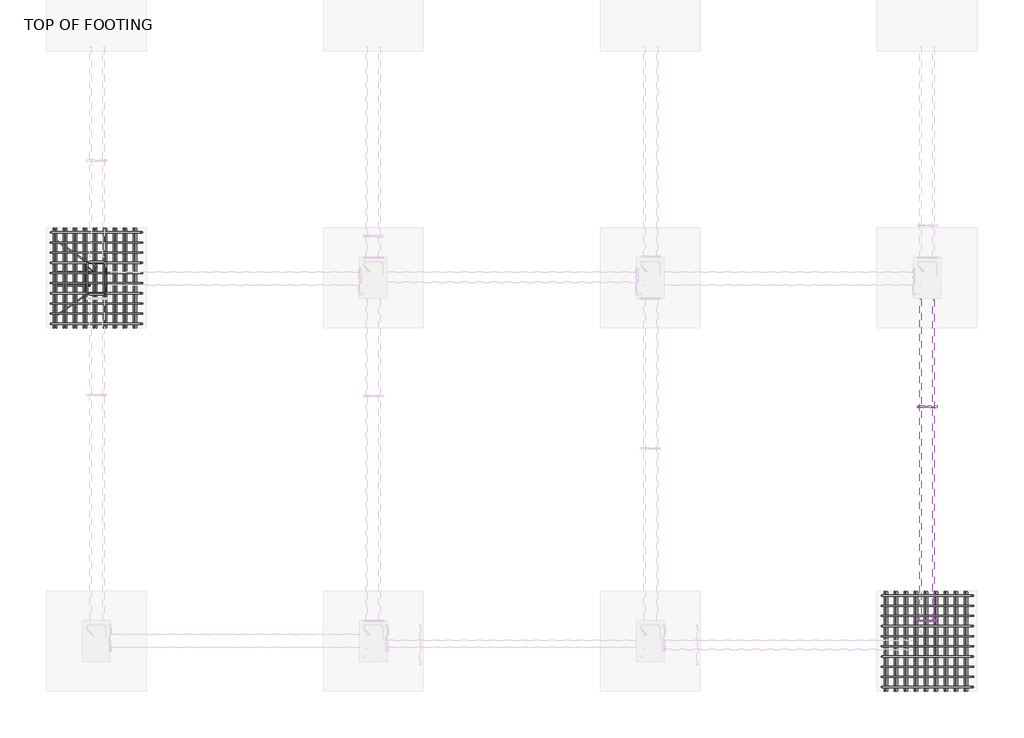
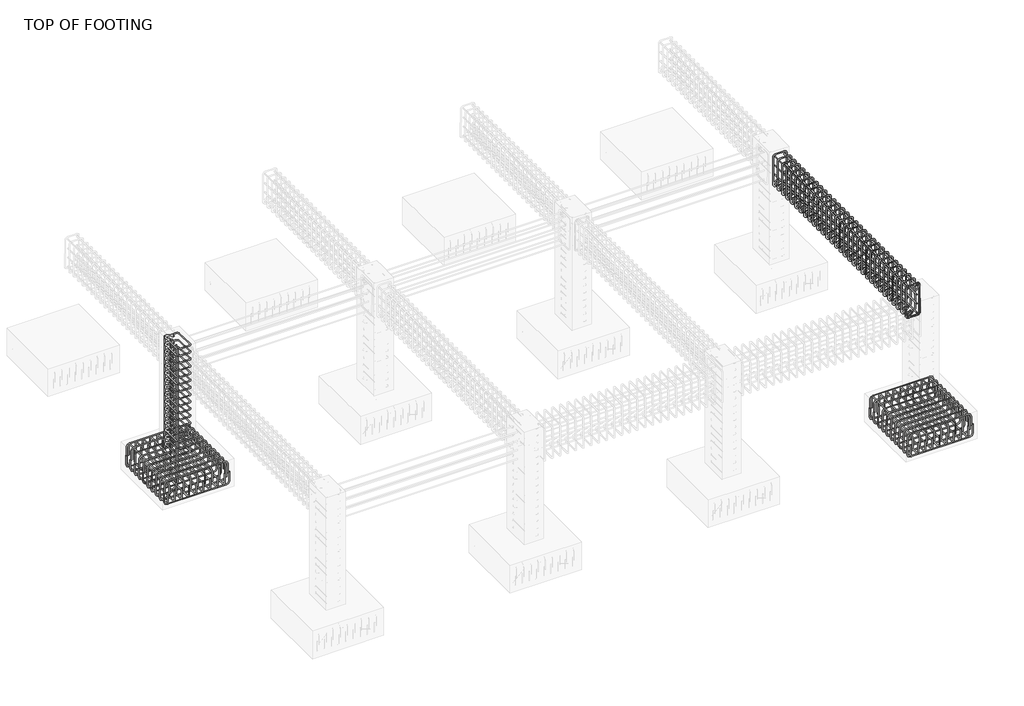
# One storey, part 5 of 18: 17 reinforcing bars.
"""IFC4 building model written with IfcOpenShell, lengths in millimetres."""

from ifc_helpers import new_model, si_unit, point, frame, origin, place, context, project, spatial, polyline, circle_curve, trimmed, segment, composite_curve, source, transform, mapped, element, save
from ifc_brep_helpers import swept_disk

model = new_model("IFC4")

# Units and contexts
model_context = context("Model", 3, world=origin())
ifc_project = project(units=[si_unit("LENGTHUNIT", "METRE", prefix="MILLI")], contexts=[model_context])

# Site, building, storey
site = spatial("IfcSite", under=ifc_project)
building = spatial("IfcBuilding", under=site)
storey = spatial("IfcBuildingStorey", under=building, Name="TOP OF FOOTING", Elevation=-1828.8)

# Reinforcing bars
placement = place(None, origin())
reinforcing_bar_shape = source(origin(), model_context, "Body", "SolidModel", [
    swept_disk(composite_curve([segment(polyline([(-11115.9859643, 9574.8477614, -40.0), (-11115.9859643, 9574.8477614, -2185.2530621)]), True, "CONTINUOUS"), segment(trimmed(circle_curve(frame((-11162.3359643, 9574.8477614, -2185.2530621), z_axis=(0.0, 1.0, 0.0), x_axis=(46.350000000000364, 0.0, 0.0)), 46.35), [point((-11115.9859643, 9574.8477614, -2185.2530621))], [point((-11162.3359643, 9574.8477614, -2231.6030621))], True, "CARTESIAN"), True, "CONTINUOUS"), segment(polyline([(-11162.3359643, 9574.8477614, -2231.6030621), (-11513.5126143, 9574.8477614, -2231.6030621)]), True, "CONTINUOUS")], self_intersect=False), 6.35),
])
element("IfcReinforcingBar", 1, at=placement, inside=storey, context=model_context, shape_type="MappedRepresentation", body=[
    mapped(reinforcing_bar_shape, transform((0.0, 0.0, 0.0), x_axis=(1.0, 0.0, 0.0), y_axis=(0.0, 1.0, 0.0), z_axis=(0.0, 0.0, 1.0))),
    mapped(reinforcing_bar_shape, transform((0.0, 148.3194112, 0.0), x_axis=(1.0, 0.0, 0.0), y_axis=(0.0, 1.0, 0.0), z_axis=(0.0, 0.0, 1.0))),
])
element("IfcReinforcingBar", 2, at=placement, inside=storey, context=model_context, shape_type="SolidModel", body=[
    swept_disk(composite_curve([segment(polyline([(-11140.9859643, 9830.3098681, -40.0), (-11140.9859643, 9830.3098681, -2185.2530621)]), True, "CONTINUOUS"), segment(trimmed(circle_curve(frame((-11178.9536616, 9856.895136, -2185.2530621), z_axis=(0.5735764363510552, 0.8191520442889855, 0.0), x_axis=(37.96769730000051, -26.585267899999963, 0.0)), 46.35), [point((-11140.9859643, 9830.3098681, -2185.2530621))], [point((-11178.9536616, 9856.895136, -2231.6030621))], True, "CARTESIAN"), True, "CONTINUOUS"), segment(polyline([(-11178.9536616, 9856.895136, -2231.6030621), (-11466.6207323, 10058.3217874, -2231.6030621)]), True, "CONTINUOUS")], self_intersect=False), 6.35),
])
reinforcing_bar_2_shape = source(origin(), model_context, "Body", "SolidModel", [
    swept_disk(composite_curve([segment(polyline([(-11036.6954038, 9770.3841028, -1782.45), (-11092.4389667, 9826.1276657, -1782.45)]), True, "CONTINUOUS"), segment(trimmed(circle_curve(frame((-11114.6067643, 9803.9598681, -1782.45), z_axis=(0.0, 0.0, 1.0), x_axis=(22.167797600000995, 22.167797599999176, 0.0)), 31.35), [point((-11092.4389667, 9826.1276657, -1782.45))], [point((-11145.9567643, 9803.9598681, -1782.45))], True, "CARTESIAN"), True, "CONTINUOUS"), segment(polyline([(-11145.9567643, 9803.9598681, -1782.45), (-11145.9567643, 9509.3598681, -1782.45)]), True, "CONTINUOUS"), segment(trimmed(circle_curve(frame((-11114.6067643, 9509.3598681, -1782.45), z_axis=(0.0, 0.0, 1.0), x_axis=(-31.349999999998545, 0.0, 0.0)), 31.35), [point((-11145.9567643, 9509.3598681, -1782.45))], [point((-11114.6067643, 9478.0098681, -1782.45))], True, "CARTESIAN"), True, "CONTINUOUS"), segment(polyline([(-11114.6067643, 9478.0098681, -1782.45), (-10970.0067643, 9478.0098681, -1782.45)]), True, "CONTINUOUS"), segment(trimmed(circle_curve(frame((-10970.0067643, 9509.3400831, -1783.5636125), z_axis=(0.0, 0.03552192833448201, 0.9993688971583016), x_axis=(0.0, -31.330214999999953, 1.1136125000000447)), 31.35), [point((-10970.0067643, 9478.0098681, -1782.45))], [point((-10938.6567643, 9509.3400831, -1783.5636125))], True, "CARTESIAN"), True, "CONTINUOUS"), segment(polyline([(-10938.6567643, 9509.3400831, -1783.5636125), (-10938.6567643, 9803.9796532, -1794.0363875)]), True, "CONTINUOUS"), segment(trimmed(circle_curve(frame((-10970.0067643, 9803.9796532, -1794.0363875), z_axis=(0.0, 0.03552192833448201, 0.9993688971583016), x_axis=(31.350000000000364, 0.0, 0.0)), 31.35), [point((-10938.6567643, 9803.9796532, -1794.0363875))], [point((-10970.0067643, 9835.3098681, -1795.15))], True, "CARTESIAN"), True, "CONTINUOUS"), segment(polyline([(-10970.0067643, 9835.3098681, -1795.15), (-11114.6067643, 9835.3098681, -1795.15)]), True, "CONTINUOUS"), segment(trimmed(circle_curve(frame((-11114.6067643, 9803.9598681, -1795.15), z_axis=(0.0, 0.0, 1.0), x_axis=(0.0, 31.349999999998545, 0.0)), 31.35), [point((-11114.6067643, 9835.3098681, -1795.15))], [point((-11136.7745619, 9781.7920705, -1795.15))], True, "CARTESIAN"), True, "CONTINUOUS"), segment(polyline([(-11136.7745619, 9781.7920705, -1795.15), (-11081.030999, 9726.0485076, -1795.15)]), True, "CONTINUOUS")], self_intersect=False), 6.35),
])
element("IfcReinforcingBar", 3, at=placement, inside=storey, context=model_context, shape_type="MappedRepresentation", body=[
    mapped(reinforcing_bar_2_shape, transform((0.0, 0.0, 0.0), x_axis=(1.0, 0.0, 0.0), y_axis=(0.0, 1.0, 0.0), z_axis=(0.0, 0.0, 1.0))),
    mapped(reinforcing_bar_2_shape, transform((0.0, 0.0, 116.0092918), x_axis=(1.0, 0.0, 0.0), y_axis=(0.0, 1.0, 0.0), z_axis=(0.0, 0.0, 1.0))),
    mapped(reinforcing_bar_2_shape, transform((0.0, 0.0, 232.0185836), x_axis=(1.0, 0.0, 0.0), y_axis=(0.0, 1.0, 0.0), z_axis=(0.0, 0.0, 1.0))),
    mapped(reinforcing_bar_2_shape, transform((0.0, 0.0, 348.0278755), x_axis=(1.0, 0.0, 0.0), y_axis=(0.0, 1.0, 0.0), z_axis=(0.0, 0.0, 1.0))),
    mapped(reinforcing_bar_2_shape, transform((0.0, 0.0, 464.0371673), x_axis=(1.0, 0.0, 0.0), y_axis=(0.0, 1.0, 0.0), z_axis=(0.0, 0.0, 1.0))),
    mapped(reinforcing_bar_2_shape, transform((0.0, 0.0, 580.0464591), x_axis=(1.0, 0.0, 0.0), y_axis=(0.0, 1.0, 0.0), z_axis=(0.0, 0.0, 1.0))),
    mapped(reinforcing_bar_2_shape, transform((0.0, 0.0, 696.0557509), x_axis=(1.0, 0.0, 0.0), y_axis=(0.0, 1.0, 0.0), z_axis=(0.0, 0.0, 1.0))),
    mapped(reinforcing_bar_2_shape, transform((0.0, 0.0, 812.0650428), x_axis=(1.0, 0.0, 0.0), y_axis=(0.0, 1.0, 0.0), z_axis=(0.0, 0.0, 1.0))),
    mapped(reinforcing_bar_2_shape, transform((0.0, 0.0, 928.0743346), x_axis=(1.0, 0.0, 0.0), y_axis=(0.0, 1.0, 0.0), z_axis=(0.0, 0.0, 1.0))),
    mapped(reinforcing_bar_2_shape, transform((0.0, 0.0, 1044.0836264), x_axis=(1.0, 0.0, 0.0), y_axis=(0.0, 1.0, 0.0), z_axis=(0.0, 0.0, 1.0))),
    mapped(reinforcing_bar_2_shape, transform((0.0, 0.0, 1160.0929182), x_axis=(1.0, 0.0, 0.0), y_axis=(0.0, 1.0, 0.0), z_axis=(0.0, 0.0, 1.0))),
    mapped(reinforcing_bar_2_shape, transform((0.0, 0.0, 1276.1022101), x_axis=(1.0, 0.0, 0.0), y_axis=(0.0, 1.0, 0.0), z_axis=(0.0, 0.0, 1.0))),
    mapped(reinforcing_bar_2_shape, transform((0.0, 0.0, 1392.1115019), x_axis=(1.0, 0.0, 0.0), y_axis=(0.0, 1.0, 0.0), z_axis=(0.0, 0.0, 1.0))),
    mapped(reinforcing_bar_2_shape, transform((0.0, 0.0, 1508.1207937), x_axis=(1.0, 0.0, 0.0), y_axis=(0.0, 1.0, 0.0), z_axis=(0.0, 0.0, 1.0))),
    mapped(reinforcing_bar_2_shape, transform((0.0, 0.0, 1624.1300855), x_axis=(1.0, 0.0, 0.0), y_axis=(0.0, 1.0, 0.0), z_axis=(0.0, 0.0, 1.0))),
    mapped(reinforcing_bar_2_shape, transform((0.0, 0.0, 1740.1393774), x_axis=(1.0, 0.0, 0.0), y_axis=(0.0, 1.0, 0.0), z_axis=(0.0, 0.0, 1.0))),
])
element("IfcReinforcingBar", 4, at=placement, inside=storey, context=model_context, shape_type="SolidModel", body=[
    swept_disk(composite_curve([segment(polyline([(-11140.9859643, 9483.0098681, -40.0), (-11140.9859643, 9483.0098681, -2185.2530621)]), True, "CONTINUOUS"), segment(trimmed(circle_curve(frame((-11178.9536616, 9456.4246003, -2185.2530621), z_axis=(-0.5735764363510106, 0.8191520442890168, 0.0), x_axis=(37.96769730000051, 26.5852677999992, 0.0)), 46.35), [point((-11140.9859643, 9483.0098681, -2185.2530621))], [point((-11178.9536616, 9456.4246003, -2231.6030621))], True, "CARTESIAN"), True, "CONTINUOUS"), segment(polyline([(-11178.9536616, 9456.4246003, -2231.6030621), (-11466.6207323, 9254.9979489, -2231.6030621)]), True, "CONTINUOUS")], self_intersect=False), 6.35),
])
reinforcing_bar_3_shape = source(origin(), model_context, "Body", "SolidModel", [
    swept_disk(composite_curve([segment(polyline([(-1394.6567643, 6160.3098681, -2046.8654906), (-1394.6567643, 6160.3098681, -2194.1654906)]), True, "CONTINUOUS"), segment(trimmed(circle_curve(frame((-1441.0067643, 6160.3098681, -2194.1654906), z_axis=(0.0, 1.0, 0.0), x_axis=(46.34999999999991, 0.0, 0.0)), 46.35), [point((-1394.6567643, 6160.3098681, -2194.1654906))], [point((-1441.0067643, 6160.3098681, -2240.5154906))], True, "CARTESIAN"), True, "CONTINUOUS"), segment(polyline([(-1441.0067643, 6160.3098681, -2240.5154906), (-2355.6067643, 6160.3098681, -2240.5154906)]), True, "CONTINUOUS"), segment(trimmed(circle_curve(frame((-2355.6067643, 6160.3098681, -2194.1654906), z_axis=(0.0, 1.0, 0.0), x_axis=(0.0, 0.0, -46.34999999999991)), 46.35), [point((-2355.6067643, 6160.3098681, -2240.5154906))], [point((-2401.9567643, 6160.3098681, -2194.1654906))], True, "CARTESIAN"), True, "CONTINUOUS"), segment(polyline([(-2401.9567643, 6160.3098681, -2194.1654906), (-2401.9567643, 6160.3098681, -2046.8654906)]), True, "CONTINUOUS")], self_intersect=False), 6.35),
])
element("IfcReinforcingBar", 5, at=placement, inside=storey, context=model_context, shape_type="MappedRepresentation", body=[
    mapped(reinforcing_bar_3_shape, transform((0.0, 0.0, 0.0), x_axis=(1.0, 0.0, 0.0), y_axis=(0.0, 1.0, 0.0), z_axis=(0.0, 0.0, 1.0))),
    mapped(reinforcing_bar_3_shape, transform((0.0, -111.9222222, 0.0), x_axis=(1.0, 0.0, 0.0), y_axis=(0.0, 1.0, 0.0), z_axis=(0.0, 0.0, 1.0))),
    mapped(reinforcing_bar_3_shape, transform((0.0, -223.8444444, 0.0), x_axis=(1.0, 0.0, 0.0), y_axis=(0.0, 1.0, 0.0), z_axis=(0.0, 0.0, 1.0))),
    mapped(reinforcing_bar_3_shape, transform((0.0, -335.7666667, 0.0), x_axis=(1.0, 0.0, 0.0), y_axis=(0.0, 1.0, 0.0), z_axis=(0.0, 0.0, 1.0))),
    mapped(reinforcing_bar_3_shape, transform((0.0, -447.6888889, 0.0), x_axis=(1.0, 0.0, 0.0), y_axis=(0.0, 1.0, 0.0), z_axis=(0.0, 0.0, 1.0))),
    mapped(reinforcing_bar_3_shape, transform((0.0, -559.6111111, 0.0), x_axis=(1.0, 0.0, 0.0), y_axis=(0.0, 1.0, 0.0), z_axis=(0.0, 0.0, 1.0))),
    mapped(reinforcing_bar_3_shape, transform((0.0, -671.5333333, 0.0), x_axis=(1.0, 0.0, 0.0), y_axis=(0.0, 1.0, 0.0), z_axis=(0.0, 0.0, 1.0))),
    mapped(reinforcing_bar_3_shape, transform((0.0, -783.4555556, 0.0), x_axis=(1.0, 0.0, 0.0), y_axis=(0.0, 1.0, 0.0), z_axis=(0.0, 0.0, 1.0))),
    mapped(reinforcing_bar_3_shape, transform((0.0, -895.3777778, 0.0), x_axis=(1.0, 0.0, 0.0), y_axis=(0.0, 1.0, 0.0), z_axis=(0.0, 0.0, 1.0))),
    mapped(reinforcing_bar_3_shape, transform((0.0, -1007.3, 0.0), x_axis=(1.0, 0.0, 0.0), y_axis=(0.0, 1.0, 0.0), z_axis=(0.0, 0.0, 1.0))),
])
reinforcing_bar_4_shape = source(origin(), model_context, "Body", "SolidModel", [
    swept_disk(composite_curve([segment(polyline([(-2392.4399078, 6160.3098681, -2056.7800629), (-2392.4399078, 6160.3098681, -1909.4800629)]), True, "CONTINUOUS"), segment(trimmed(circle_curve(frame((-2346.0899078, 6160.3098681, -1909.4800629), z_axis=(0.0, 1.0, 0.0), x_axis=(-46.34999999999991, 0.0, 0.0)), 46.35), [point((-2392.4399078, 6160.3098681, -1909.4800629))], [point((-2346.0899078, 6160.3098681, -1863.1300629))], True, "CARTESIAN"), True, "CONTINUOUS"), segment(polyline([(-2346.0899078, 6160.3098681, -1863.1300629), (-1466.3320898, 6160.3098681, -1863.1300629)]), True, "CONTINUOUS"), segment(trimmed(circle_curve(frame((-1466.3320898, 6160.3098681, -1909.4800629), z_axis=(0.0, 1.0, 0.0), x_axis=(0.0, 0.0, 46.34999999999991)), 46.35), [point((-1466.3320898, 6160.3098681, -1863.1300629))], [point((-1419.9820898, 6160.3098681, -1909.4800629))], True, "CARTESIAN"), True, "CONTINUOUS"), segment(polyline([(-1419.9820898, 6160.3098681, -1909.4800629), (-1419.9820898, 6160.3098681, -2056.7800629)]), True, "CONTINUOUS")], self_intersect=False), 6.35),
])
element("IfcReinforcingBar", 6, at=placement, inside=storey, context=model_context, shape_type="MappedRepresentation", body=[
    mapped(reinforcing_bar_4_shape, transform((0.0, 0.0, 0.0), x_axis=(1.0, 0.0, 0.0), y_axis=(0.0, 1.0, 0.0), z_axis=(0.0, 0.0, 1.0))),
    mapped(reinforcing_bar_4_shape, transform((0.0, -111.9222222, 0.0), x_axis=(1.0, 0.0, 0.0), y_axis=(0.0, 1.0, 0.0), z_axis=(0.0, 0.0, 1.0))),
    mapped(reinforcing_bar_4_shape, transform((0.0, -223.8444444, 0.0), x_axis=(1.0, 0.0, 0.0), y_axis=(0.0, 1.0, 0.0), z_axis=(0.0, 0.0, 1.0))),
    mapped(reinforcing_bar_4_shape, transform((0.0, -335.7666667, 0.0), x_axis=(1.0, 0.0, 0.0), y_axis=(0.0, 1.0, 0.0), z_axis=(0.0, 0.0, 1.0))),
    mapped(reinforcing_bar_4_shape, transform((0.0, -447.6888889, 0.0), x_axis=(1.0, 0.0, 0.0), y_axis=(0.0, 1.0, 0.0), z_axis=(0.0, 0.0, 1.0))),
    mapped(reinforcing_bar_4_shape, transform((0.0, -559.6111111, 0.0), x_axis=(1.0, 0.0, 0.0), y_axis=(0.0, 1.0, 0.0), z_axis=(0.0, 0.0, 1.0))),
    mapped(reinforcing_bar_4_shape, transform((0.0, -671.5333333, 0.0), x_axis=(1.0, 0.0, 0.0), y_axis=(0.0, 1.0, 0.0), z_axis=(0.0, 0.0, 1.0))),
    mapped(reinforcing_bar_4_shape, transform((0.0, -783.4555556, 0.0), x_axis=(1.0, 0.0, 0.0), y_axis=(0.0, 1.0, 0.0), z_axis=(0.0, 0.0, 1.0))),
    mapped(reinforcing_bar_4_shape, transform((0.0, -895.3777778, 0.0), x_axis=(1.0, 0.0, 0.0), y_axis=(0.0, 1.0, 0.0), z_axis=(0.0, 0.0, 1.0))),
    mapped(reinforcing_bar_4_shape, transform((0.0, -1007.3, 0.0), x_axis=(1.0, 0.0, 0.0), y_axis=(0.0, 1.0, 0.0), z_axis=(0.0, 0.0, 1.0))),
])
reinforcing_bar_5_shape = source(origin(), model_context, "Body", "SolidModel", [
    swept_disk(composite_curve([segment(polyline([(-1463.1065918, 6200.3098681, -2080.1793981), (-1463.1065918, 6200.3098681, -1932.8793981)]), True, "CONTINUOUS"), segment(trimmed(circle_curve(frame((-1463.1065918, 6153.9598681, -1932.8793981), z_axis=(1.0, 0.0, 0.0), x_axis=(0.0, 46.350000000000364, 0.0)), 46.35), [point((-1463.1065918, 6200.3098681, -1932.8793981))], [point((-1463.1065918, 6153.9598681, -1886.5293981))], True, "CARTESIAN"), True, "CONTINUOUS"), segment(polyline([(-1463.1065918, 6153.9598681, -1886.5293981), (-1463.1065918, 5159.3598681, -1886.5293981)]), True, "CONTINUOUS"), segment(trimmed(circle_curve(frame((-1463.1065918, 5159.3598681, -1932.8793981), z_axis=(1.0, 0.0, 0.0), x_axis=(0.0, 0.0, 46.34999999999991)), 46.35), [point((-1463.1065918, 5159.3598681, -1886.5293981))], [point((-1463.1065918, 5113.0098681, -1932.8793981))], True, "CARTESIAN"), True, "CONTINUOUS"), segment(polyline([(-1463.1065918, 5113.0098681, -1932.8793981), (-1463.1065918, 5113.0098681, -2080.1793981)]), True, "CONTINUOUS")], self_intersect=False), 6.35),
])
element("IfcReinforcingBar", 7, at=placement, inside=storey, context=model_context, shape_type="MappedRepresentation", body=[
    mapped(reinforcing_bar_5_shape, transform((0.0, 0.0, 0.0), x_axis=(1.0, 0.0, 0.0), y_axis=(0.0, 1.0, 0.0), z_axis=(0.0, 0.0, 1.0))),
    mapped(reinforcing_bar_5_shape, transform((-109.9785589, 0.0, 0.0), x_axis=(1.0, 0.0, 0.0), y_axis=(0.0, 1.0, 0.0), z_axis=(0.0, 0.0, 1.0))),
    mapped(reinforcing_bar_5_shape, transform((-219.9571177, 0.0, 0.0), x_axis=(1.0, 0.0, 0.0), y_axis=(0.0, 1.0, 0.0), z_axis=(0.0, 0.0, 1.0))),
    mapped(reinforcing_bar_5_shape, transform((-329.9356766, 0.0, 0.0), x_axis=(1.0, 0.0, 0.0), y_axis=(0.0, 1.0, 0.0), z_axis=(0.0, 0.0, 1.0))),
    mapped(reinforcing_bar_5_shape, transform((-439.9142355, 0.0, 0.0), x_axis=(1.0, 0.0, 0.0), y_axis=(0.0, 1.0, 0.0), z_axis=(0.0, 0.0, 1.0))),
    mapped(reinforcing_bar_5_shape, transform((-549.8927943, 0.0, 0.0), x_axis=(1.0, 0.0, 0.0), y_axis=(0.0, 1.0, 0.0), z_axis=(0.0, 0.0, 1.0))),
    mapped(reinforcing_bar_5_shape, transform((-659.8713532, 0.0, 0.0), x_axis=(1.0, 0.0, 0.0), y_axis=(0.0, 1.0, 0.0), z_axis=(0.0, 0.0, 1.0))),
    mapped(reinforcing_bar_5_shape, transform((-769.8499121, 0.0, 0.0), x_axis=(1.0, 0.0, 0.0), y_axis=(0.0, 1.0, 0.0), z_axis=(0.0, 0.0, 1.0))),
    mapped(reinforcing_bar_5_shape, transform((-879.828471, 0.0, 0.0), x_axis=(1.0, 0.0, 0.0), y_axis=(0.0, 1.0, 0.0), z_axis=(0.0, 0.0, 1.0))),
])
reinforcing_bar_6_shape = source(origin(), model_context, "Body", "SolidModel", [
    swept_disk(composite_curve([segment(polyline([(-2369.5126143, 6200.3098681, -2025.2530621), (-2369.5126143, 6200.3098681, -2172.5530621)]), True, "CONTINUOUS"), segment(trimmed(circle_curve(frame((-2369.5126143, 6153.9598681, -2172.5530621), z_axis=(-1.0, 0.0, 0.0), x_axis=(0.0, 46.350000000000364, 0.0)), 46.35), [point((-2369.5126143, 6200.3098681, -2172.5530621))], [point((-2369.5126143, 6153.9598681, -2218.9030621))], True, "CARTESIAN"), True, "CONTINUOUS"), segment(polyline([(-2369.5126143, 6153.9598681, -2218.9030621), (-2369.5126143, 5159.3598681, -2218.9030621)]), True, "CONTINUOUS"), segment(trimmed(circle_curve(frame((-2369.5126143, 5159.3598681, -2172.5530621), z_axis=(-1.0, 0.0, 0.0), x_axis=(0.0, 0.0, -46.350000000000364)), 46.35), [point((-2369.5126143, 5159.3598681, -2218.9030621))], [point((-2369.5126143, 5113.0098681, -2172.5530621))], True, "CARTESIAN"), True, "CONTINUOUS"), segment(polyline([(-2369.5126143, 5113.0098681, -2172.5530621), (-2369.5126143, 5113.0098681, -2025.2530621)]), True, "CONTINUOUS")], self_intersect=False), 6.35),
])
element("IfcReinforcingBar", 8, at=placement, inside=storey, context=model_context, shape_type="MappedRepresentation", body=[
    mapped(reinforcing_bar_6_shape, transform((0.0, 0.0, 0.0), x_axis=(1.0, 0.0, 0.0), y_axis=(0.0, 1.0, 0.0), z_axis=(0.0, 0.0, 1.0))),
    mapped(reinforcing_bar_6_shape, transform((109.9890349, 0.0, 0.0), x_axis=(1.0, 0.0, 0.0), y_axis=(0.0, 1.0, 0.0), z_axis=(0.0, 0.0, 1.0))),
    mapped(reinforcing_bar_6_shape, transform((219.9780699, 0.0, 0.0), x_axis=(1.0, 0.0, 0.0), y_axis=(0.0, 1.0, 0.0), z_axis=(0.0, 0.0, 1.0))),
    mapped(reinforcing_bar_6_shape, transform((329.9671048, 0.0, 0.0), x_axis=(1.0, 0.0, 0.0), y_axis=(0.0, 1.0, 0.0), z_axis=(0.0, 0.0, 1.0))),
    mapped(reinforcing_bar_6_shape, transform((439.9561397, 0.0, 0.0), x_axis=(1.0, 0.0, 0.0), y_axis=(0.0, 1.0, 0.0), z_axis=(0.0, 0.0, 1.0))),
    mapped(reinforcing_bar_6_shape, transform((549.9451746, 0.0, 0.0), x_axis=(1.0, 0.0, 0.0), y_axis=(0.0, 1.0, 0.0), z_axis=(0.0, 0.0, 1.0))),
    mapped(reinforcing_bar_6_shape, transform((659.9342096, 0.0, 0.0), x_axis=(1.0, 0.0, 0.0), y_axis=(0.0, 1.0, 0.0), z_axis=(0.0, 0.0, 1.0))),
    mapped(reinforcing_bar_6_shape, transform((769.9232445, 0.0, 0.0), x_axis=(1.0, 0.0, 0.0), y_axis=(0.0, 1.0, 0.0), z_axis=(0.0, 0.0, 1.0))),
    mapped(reinforcing_bar_6_shape, transform((879.9122794, 0.0, 0.0), x_axis=(1.0, 0.0, 0.0), y_axis=(0.0, 1.0, 0.0), z_axis=(0.0, 0.0, 1.0))),
])
reinforcing_bar_7_shape = source(origin(), model_context, "Body", "SolidModel", [
    swept_disk(composite_curve([segment(polyline([(-10538.6567643, 10160.3098681, -2046.8654906), (-10538.6567643, 10160.3098681, -2194.1654906)]), True, "CONTINUOUS"), segment(trimmed(circle_curve(frame((-10585.0067643, 10160.3098681, -2194.1654906), z_axis=(0.0, 1.0, 0.0), x_axis=(46.350000000000364, 0.0, 0.0)), 46.35), [point((-10538.6567643, 10160.3098681, -2194.1654906))], [point((-10585.0067643, 10160.3098681, -2240.5154906))], True, "CARTESIAN"), True, "CONTINUOUS"), segment(polyline([(-10585.0067643, 10160.3098681, -2240.5154906), (-11499.6067643, 10160.3098681, -2240.5154906)]), True, "CONTINUOUS"), segment(trimmed(circle_curve(frame((-11499.6067643, 10160.3098681, -2194.1654906), z_axis=(0.0, 1.0, 0.0), x_axis=(0.0, 0.0, -46.34999999999991)), 46.35), [point((-11499.6067643, 10160.3098681, -2240.5154906))], [point((-11545.9567643, 10160.3098681, -2194.1654906))], True, "CARTESIAN"), True, "CONTINUOUS"), segment(polyline([(-11545.9567643, 10160.3098681, -2194.1654906), (-11545.9567643, 10160.3098681, -2046.8654906)]), True, "CONTINUOUS")], self_intersect=False), 6.35),
])
element("IfcReinforcingBar", 9, at=placement, inside=storey, context=model_context, shape_type="MappedRepresentation", body=[
    mapped(reinforcing_bar_7_shape, transform((0.0, 0.0, 0.0), x_axis=(1.0, 0.0, 0.0), y_axis=(0.0, 1.0, 0.0), z_axis=(0.0, 0.0, 1.0))),
    mapped(reinforcing_bar_7_shape, transform((0.0, -111.9222222, 0.0), x_axis=(1.0, 0.0, 0.0), y_axis=(0.0, 1.0, 0.0), z_axis=(0.0, 0.0, 1.0))),
    mapped(reinforcing_bar_7_shape, transform((0.0, -223.8444444, 0.0), x_axis=(1.0, 0.0, 0.0), y_axis=(0.0, 1.0, 0.0), z_axis=(0.0, 0.0, 1.0))),
    mapped(reinforcing_bar_7_shape, transform((0.0, -335.7666667, 0.0), x_axis=(1.0, 0.0, 0.0), y_axis=(0.0, 1.0, 0.0), z_axis=(0.0, 0.0, 1.0))),
    mapped(reinforcing_bar_7_shape, transform((0.0, -447.6888889, 0.0), x_axis=(1.0, 0.0, 0.0), y_axis=(0.0, 1.0, 0.0), z_axis=(0.0, 0.0, 1.0))),
    mapped(reinforcing_bar_7_shape, transform((0.0, -559.6111111, 0.0), x_axis=(1.0, 0.0, 0.0), y_axis=(0.0, 1.0, 0.0), z_axis=(0.0, 0.0, 1.0))),
    mapped(reinforcing_bar_7_shape, transform((0.0, -671.5333333, 0.0), x_axis=(1.0, 0.0, 0.0), y_axis=(0.0, 1.0, 0.0), z_axis=(0.0, 0.0, 1.0))),
    mapped(reinforcing_bar_7_shape, transform((0.0, -783.4555556, 0.0), x_axis=(1.0, 0.0, 0.0), y_axis=(0.0, 1.0, 0.0), z_axis=(0.0, 0.0, 1.0))),
    mapped(reinforcing_bar_7_shape, transform((0.0, -895.3777778, 0.0), x_axis=(1.0, 0.0, 0.0), y_axis=(0.0, 1.0, 0.0), z_axis=(0.0, 0.0, 1.0))),
    mapped(reinforcing_bar_7_shape, transform((0.0, -1007.3, 0.0), x_axis=(1.0, 0.0, 0.0), y_axis=(0.0, 1.0, 0.0), z_axis=(0.0, 0.0, 1.0))),
])
reinforcing_bar_8_shape = source(origin(), model_context, "Body", "SolidModel", [
    swept_disk(composite_curve([segment(polyline([(-11536.4399078, 10160.3098681, -2056.7800629), (-11536.4399078, 10160.3098681, -1909.4800629)]), True, "CONTINUOUS"), segment(trimmed(circle_curve(frame((-11490.0899078, 10160.3098681, -1909.4800629), z_axis=(0.0, 1.0, 0.0), x_axis=(-46.350000000000364, 0.0, 0.0)), 46.35), [point((-11536.4399078, 10160.3098681, -1909.4800629))], [point((-11490.0899078, 10160.3098681, -1863.1300629))], True, "CARTESIAN"), True, "CONTINUOUS"), segment(polyline([(-11490.0899078, 10160.3098681, -1863.1300629), (-10610.3320898, 10160.3098681, -1863.1300629)]), True, "CONTINUOUS"), segment(trimmed(circle_curve(frame((-10610.3320898, 10160.3098681, -1909.4800629), z_axis=(0.0, 1.0, 0.0), x_axis=(0.0, 0.0, 46.34999999999991)), 46.35), [point((-10610.3320898, 10160.3098681, -1863.1300629))], [point((-10563.9820898, 10160.3098681, -1909.4800629))], True, "CARTESIAN"), True, "CONTINUOUS"), segment(polyline([(-10563.9820898, 10160.3098681, -1909.4800629), (-10563.9820898, 10160.3098681, -2056.7800629)]), True, "CONTINUOUS")], self_intersect=False), 6.35),
])
element("IfcReinforcingBar", 10, at=placement, inside=storey, context=model_context, shape_type="MappedRepresentation", body=[
    mapped(reinforcing_bar_8_shape, transform((0.0, 0.0, 0.0), x_axis=(1.0, 0.0, 0.0), y_axis=(0.0, 1.0, 0.0), z_axis=(0.0, 0.0, 1.0))),
    mapped(reinforcing_bar_8_shape, transform((0.0, -111.9222222, 0.0), x_axis=(1.0, 0.0, 0.0), y_axis=(0.0, 1.0, 0.0), z_axis=(0.0, 0.0, 1.0))),
    mapped(reinforcing_bar_8_shape, transform((0.0, -223.8444444, 0.0), x_axis=(1.0, 0.0, 0.0), y_axis=(0.0, 1.0, 0.0), z_axis=(0.0, 0.0, 1.0))),
    mapped(reinforcing_bar_8_shape, transform((0.0, -335.7666667, 0.0), x_axis=(1.0, 0.0, 0.0), y_axis=(0.0, 1.0, 0.0), z_axis=(0.0, 0.0, 1.0))),
    mapped(reinforcing_bar_8_shape, transform((0.0, -447.6888889, 0.0), x_axis=(1.0, 0.0, 0.0), y_axis=(0.0, 1.0, 0.0), z_axis=(0.0, 0.0, 1.0))),
    mapped(reinforcing_bar_8_shape, transform((0.0, -559.6111111, 0.0), x_axis=(1.0, 0.0, 0.0), y_axis=(0.0, 1.0, 0.0), z_axis=(0.0, 0.0, 1.0))),
    mapped(reinforcing_bar_8_shape, transform((0.0, -671.5333333, 0.0), x_axis=(1.0, 0.0, 0.0), y_axis=(0.0, 1.0, 0.0), z_axis=(0.0, 0.0, 1.0))),
    mapped(reinforcing_bar_8_shape, transform((0.0, -783.4555556, 0.0), x_axis=(1.0, 0.0, 0.0), y_axis=(0.0, 1.0, 0.0), z_axis=(0.0, 0.0, 1.0))),
    mapped(reinforcing_bar_8_shape, transform((0.0, -895.3777778, 0.0), x_axis=(1.0, 0.0, 0.0), y_axis=(0.0, 1.0, 0.0), z_axis=(0.0, 0.0, 1.0))),
    mapped(reinforcing_bar_8_shape, transform((0.0, -1007.3, 0.0), x_axis=(1.0, 0.0, 0.0), y_axis=(0.0, 1.0, 0.0), z_axis=(0.0, 0.0, 1.0))),
])
reinforcing_bar_9_shape = source(origin(), model_context, "Body", "SolidModel", [
    swept_disk(composite_curve([segment(polyline([(-10607.1065918, 10200.3098681, -2080.1793981), (-10607.1065918, 10200.3098681, -1932.8793981)]), True, "CONTINUOUS"), segment(trimmed(circle_curve(frame((-10607.1065918, 10153.9598681, -1932.8793981), z_axis=(1.0, 0.0, 0.0), x_axis=(0.0, 46.349999999998545, 0.0)), 46.35), [point((-10607.1065918, 10200.3098681, -1932.8793981))], [point((-10607.1065918, 10153.9598681, -1886.5293981))], True, "CARTESIAN"), True, "CONTINUOUS"), segment(polyline([(-10607.1065918, 10153.9598681, -1886.5293981), (-10607.1065918, 9159.3598681, -1886.5293981)]), True, "CONTINUOUS"), segment(trimmed(circle_curve(frame((-10607.1065918, 9159.3598681, -1932.8793981), z_axis=(1.0, 0.0, 0.0), x_axis=(0.0, 0.0, 46.34999999999991)), 46.35), [point((-10607.1065918, 9159.3598681, -1886.5293981))], [point((-10607.1065918, 9113.0098681, -1932.8793981))], True, "CARTESIAN"), True, "CONTINUOUS"), segment(polyline([(-10607.1065918, 9113.0098681, -1932.8793981), (-10607.1065918, 9113.0098681, -2080.1793981)]), True, "CONTINUOUS")], self_intersect=False), 6.35),
])
element("IfcReinforcingBar", 11, at=placement, inside=storey, context=model_context, shape_type="MappedRepresentation", body=[
    mapped(reinforcing_bar_9_shape, transform((0.0, 0.0, 0.0), x_axis=(1.0, 0.0, 0.0), y_axis=(0.0, 1.0, 0.0), z_axis=(0.0, 0.0, 1.0))),
    mapped(reinforcing_bar_9_shape, transform((-109.9785589, 0.0, 0.0), x_axis=(1.0, 0.0, 0.0), y_axis=(0.0, 1.0, 0.0), z_axis=(0.0, 0.0, 1.0))),
    mapped(reinforcing_bar_9_shape, transform((-219.9571177, 0.0, 0.0), x_axis=(1.0, 0.0, 0.0), y_axis=(0.0, 1.0, 0.0), z_axis=(0.0, 0.0, 1.0))),
    mapped(reinforcing_bar_9_shape, transform((-329.9356766, 0.0, 0.0), x_axis=(1.0, 0.0, 0.0), y_axis=(0.0, 1.0, 0.0), z_axis=(0.0, 0.0, 1.0))),
    mapped(reinforcing_bar_9_shape, transform((-439.9142355, 0.0, 0.0), x_axis=(1.0, 0.0, 0.0), y_axis=(0.0, 1.0, 0.0), z_axis=(0.0, 0.0, 1.0))),
    mapped(reinforcing_bar_9_shape, transform((-549.8927943, 0.0, 0.0), x_axis=(1.0, 0.0, 0.0), y_axis=(0.0, 1.0, 0.0), z_axis=(0.0, 0.0, 1.0))),
    mapped(reinforcing_bar_9_shape, transform((-659.8713532, 0.0, 0.0), x_axis=(1.0, 0.0, 0.0), y_axis=(0.0, 1.0, 0.0), z_axis=(0.0, 0.0, 1.0))),
    mapped(reinforcing_bar_9_shape, transform((-769.8499121, 0.0, 0.0), x_axis=(1.0, 0.0, 0.0), y_axis=(0.0, 1.0, 0.0), z_axis=(0.0, 0.0, 1.0))),
    mapped(reinforcing_bar_9_shape, transform((-879.828471, 0.0, 0.0), x_axis=(1.0, 0.0, 0.0), y_axis=(0.0, 1.0, 0.0), z_axis=(0.0, 0.0, 1.0))),
])
reinforcing_bar_10_shape = source(origin(), model_context, "Body", "SolidModel", [
    swept_disk(composite_curve([segment(polyline([(-11513.5126143, 10200.3098681, -2025.2530621), (-11513.5126143, 10200.3098681, -2172.5530621)]), True, "CONTINUOUS"), segment(trimmed(circle_curve(frame((-11513.5126143, 10153.9598681, -2172.5530621), z_axis=(-1.0, 0.0, 0.0), x_axis=(0.0, 46.349999999998545, 0.0)), 46.35), [point((-11513.5126143, 10200.3098681, -2172.5530621))], [point((-11513.5126143, 10153.9598681, -2218.9030621))], True, "CARTESIAN"), True, "CONTINUOUS"), segment(polyline([(-11513.5126143, 10153.9598681, -2218.9030621), (-11513.5126143, 9159.3598681, -2218.9030621)]), True, "CONTINUOUS"), segment(trimmed(circle_curve(frame((-11513.5126143, 9159.3598681, -2172.5530621), z_axis=(-1.0, 0.0, 0.0), x_axis=(0.0, 0.0, -46.350000000000364)), 46.35), [point((-11513.5126143, 9159.3598681, -2218.9030621))], [point((-11513.5126143, 9113.0098681, -2172.5530621))], True, "CARTESIAN"), True, "CONTINUOUS"), segment(polyline([(-11513.5126143, 9113.0098681, -2172.5530621), (-11513.5126143, 9113.0098681, -2025.2530621)]), True, "CONTINUOUS")], self_intersect=False), 6.35),
])
element("IfcReinforcingBar", 12, at=placement, inside=storey, context=model_context, shape_type="MappedRepresentation", body=[
    mapped(reinforcing_bar_10_shape, transform((0.0, 0.0, 0.0), x_axis=(1.0, 0.0, 0.0), y_axis=(0.0, 1.0, 0.0), z_axis=(0.0, 0.0, 1.0))),
    mapped(reinforcing_bar_10_shape, transform((109.9890349, 0.0, 0.0), x_axis=(1.0, 0.0, 0.0), y_axis=(0.0, 1.0, 0.0), z_axis=(0.0, 0.0, 1.0))),
    mapped(reinforcing_bar_10_shape, transform((219.9780699, 0.0, 0.0), x_axis=(1.0, 0.0, 0.0), y_axis=(0.0, 1.0, 0.0), z_axis=(0.0, 0.0, 1.0))),
    mapped(reinforcing_bar_10_shape, transform((329.9671048, 0.0, 0.0), x_axis=(1.0, 0.0, 0.0), y_axis=(0.0, 1.0, 0.0), z_axis=(0.0, 0.0, 1.0))),
    mapped(reinforcing_bar_10_shape, transform((439.9561397, 0.0, 0.0), x_axis=(1.0, 0.0, 0.0), y_axis=(0.0, 1.0, 0.0), z_axis=(0.0, 0.0, 1.0))),
    mapped(reinforcing_bar_10_shape, transform((549.9451746, 0.0, 0.0), x_axis=(1.0, 0.0, 0.0), y_axis=(0.0, 1.0, 0.0), z_axis=(0.0, 0.0, 1.0))),
    mapped(reinforcing_bar_10_shape, transform((659.9342096, 0.0, 0.0), x_axis=(1.0, 0.0, 0.0), y_axis=(0.0, 1.0, 0.0), z_axis=(0.0, 0.0, 1.0))),
    mapped(reinforcing_bar_10_shape, transform((769.9232445, 0.0, 0.0), x_axis=(1.0, 0.0, 0.0), y_axis=(0.0, 1.0, 0.0), z_axis=(0.0, 0.0, 1.0))),
    mapped(reinforcing_bar_10_shape, transform((879.9122794, 0.0, 0.0), x_axis=(1.0, 0.0, 0.0), y_axis=(0.0, 1.0, 0.0), z_axis=(0.0, 0.0, 1.0))),
])
element("IfcReinforcingBar", 13, at=placement, inside=storey, context=model_context, shape_type="SolidModel", body=[
    swept_disk(composite_curve([segment(polyline([(-1903.9181249, 5888.0098675, -111.2757654), (-1848.1745619, 5888.0098675, -55.5322024)]), True, "CONTINUOUS"), segment(trimmed(circle_curve(frame((-1826.0067643, 5888.0098675, -77.7), z_axis=(0.0, 1.0, 0.0), x_axis=(-22.167797600000085, 0.0, 22.1677976)), 31.35), [point((-1848.1745619, 5888.0098675, -55.5322024))], [point((-1794.6567643, 5888.0098675, -77.7))], True, "CARTESIAN"), True, "CONTINUOUS"), segment(polyline([(-1794.6567643, 5888.0098675, -77.7), (-1794.6567643, 5888.0098675, -522.3)]), True, "CONTINUOUS"), segment(trimmed(circle_curve(frame((-1826.0067643, 5888.0098675, -522.3), z_axis=(0.0, 1.0, 0.0), x_axis=(31.34999999999991, 0.0, 0.0)), 31.35), [point((-1794.6567643, 5888.0098675, -522.3))], [point((-1826.0067643, 5888.0098675, -553.65))], True, "CARTESIAN"), True, "CONTINUOUS"), segment(polyline([(-1826.0067643, 5888.0098675, -553.65), (-1970.6067643, 5888.0098675, -553.65)]), True, "CONTINUOUS"), segment(trimmed(circle_curve(frame((-1970.6067643, 5887.2252819, -522.3098193), z_axis=(0.0, 0.9996867842138424, 0.025026655153786322), x_axis=(0.0, 0.784585600000355, -31.34018070000002)), 31.35), [point((-1970.6067643, 5888.0098675, -553.65))], [point((-2001.9567643, 5887.2252819, -522.3098193))], True, "CARTESIAN"), True, "CONTINUOUS"), segment(polyline([(-2001.9567643, 5887.2252819, -522.3098193), (-2001.9567643, 5876.0944532, -77.6901807)]), True, "CONTINUOUS"), segment(trimmed(circle_curve(frame((-1970.6067643, 5876.0944532, -77.6901807), z_axis=(0.0, 0.9996867842138424, 0.025026655153786322), x_axis=(-31.350000000000136, 0.0, 0.0)), 31.35), [point((-2001.9567643, 5876.0944532, -77.6901807))], [point((-1970.6067643, 5875.3098675, -46.35))], True, "CARTESIAN"), True, "CONTINUOUS"), segment(polyline([(-1970.6067643, 5875.3098675, -46.35), (-1826.0067643, 5875.3098675, -46.35)]), True, "CONTINUOUS"), segment(trimmed(circle_curve(frame((-1826.0067643, 5875.3098675, -77.7), z_axis=(0.0, 1.0, 0.0), x_axis=(0.0, 0.0, 31.35)), 31.35), [point((-1826.0067643, 5875.3098675, -46.35))], [point((-1803.8389667, 5875.3098675, -99.8677976))], True, "CARTESIAN"), True, "CONTINUOUS"), segment(polyline([(-1803.8389667, 5875.3098675, -99.8677976), (-1859.5825297, 5875.3098675, -155.6113605)]), True, "CONTINUOUS")], self_intersect=False), 6.35),
])
element("IfcReinforcingBar", 14, at=placement, inside=storey, context=model_context, shape_type="SolidModel", body=[
    swept_disk(composite_curve([segment(polyline([(-1892.6954038, 5888.0098675, -488.7242346), (-1948.4389667, 5888.0098675, -544.4677976)]), True, "CONTINUOUS"), segment(trimmed(circle_curve(frame((-1970.6067643, 5888.0098675, -522.3), z_axis=(0.0, 1.0, 0.0), x_axis=(22.167797599999858, 0.0, -22.167797600000085)), 31.35), [point((-1948.4389667, 5888.0098675, -544.4677976))], [point((-2001.9567643, 5888.0098675, -522.3))], True, "CARTESIAN"), True, "CONTINUOUS"), segment(polyline([(-2001.9567643, 5888.0098675, -522.3), (-2001.9567643, 5888.0098675, -77.7)]), True, "CONTINUOUS"), segment(trimmed(circle_curve(frame((-1970.6067643, 5888.0098675, -77.7), z_axis=(0.0, 1.0, 0.0), x_axis=(-31.350000000000136, 0.0, 0.0)), 31.35), [point((-2001.9567643, 5888.0098675, -77.7))], [point((-1970.6067643, 5888.0098675, -46.35))], True, "CARTESIAN"), True, "CONTINUOUS"), segment(polyline([(-1970.6067643, 5888.0098675, -46.35), (-1826.0067643, 5888.0098675, -46.35)]), True, "CONTINUOUS"), segment(trimmed(circle_curve(frame((-1826.0067643, 5887.2252819, -77.6901807), z_axis=(0.0, 0.9996867842138424, -0.025026655153786322), x_axis=(0.0, 0.784585600000355, 31.340180699999998)), 31.35), [point((-1826.0067643, 5888.0098675, -46.35))], [point((-1794.6567643, 5887.2252819, -77.6901807))], True, "CARTESIAN"), True, "CONTINUOUS"), segment(polyline([(-1794.6567643, 5887.2252819, -77.6901807), (-1794.6567643, 5876.0944532, -522.3098193)]), True, "CONTINUOUS"), segment(trimmed(circle_curve(frame((-1826.0067643, 5876.0944532, -522.3098193), z_axis=(0.0, 0.9996867842138424, -0.025026655153786322), x_axis=(31.34999999999991, 0.0, 0.0)), 31.35), [point((-1794.6567643, 5876.0944532, -522.3098193))], [point((-1826.0067643, 5875.3098675, -553.65))], True, "CARTESIAN"), True, "CONTINUOUS"), segment(polyline([(-1826.0067643, 5875.3098675, -553.65), (-1970.6067643, 5875.3098675, -553.65)]), True, "CONTINUOUS"), segment(trimmed(circle_curve(frame((-1970.6067643, 5875.3098675, -522.3), z_axis=(0.0, 1.0, 0.0), x_axis=(0.0, 0.0, -31.350000000000023)), 31.35), [point((-1970.6067643, 5875.3098675, -553.65))], [point((-1992.7745619, 5875.3098675, -500.1322024))], True, "CARTESIAN"), True, "CONTINUOUS"), segment(polyline([(-1992.7745619, 5875.3098675, -500.1322024), (-1937.030999, 5875.3098675, -444.3886395)]), True, "CONTINUOUS")], self_intersect=False), 6.35),
])
reinforcing_bar_11_shape = source(origin(), model_context, "Body", "SolidModel", [
    swept_disk(composite_curve([segment(polyline([(-1892.6954038, 5888.0098675, -488.7242346), (-1948.4389667, 5888.0098675, -544.4677976)]), True, "CONTINUOUS"), segment(trimmed(circle_curve(frame((-1970.6067643, 5888.0098675, -522.3), z_axis=(0.0, 1.0, 0.0), x_axis=(22.167797599999858, 0.0, -22.167797600000085)), 31.35), [point((-1948.4389667, 5888.0098675, -544.4677976))], [point((-2001.9567643, 5888.0098675, -522.3))], True, "CARTESIAN"), True, "CONTINUOUS"), segment(polyline([(-2001.9567643, 5888.0098675, -522.3), (-2001.9567643, 5888.0098675, -77.7)]), True, "CONTINUOUS"), segment(trimmed(circle_curve(frame((-1970.6067643, 5888.0098675, -77.7), z_axis=(0.0, 1.0, 0.0), x_axis=(-31.350000000000136, 0.0, 0.0)), 31.35), [point((-2001.9567643, 5888.0098675, -77.7))], [point((-1970.6067643, 5888.0098675, -46.35))], True, "CARTESIAN"), True, "CONTINUOUS"), segment(polyline([(-1970.6067643, 5888.0098675, -46.35), (-1826.0067643, 5888.0098675, -46.35)]), True, "CONTINUOUS"), segment(trimmed(circle_curve(frame((-1826.0067643, 5887.2252819, -77.6901807), z_axis=(0.0, 0.9996867842138424, -0.025026655153786322), x_axis=(0.0, 0.784585600000355, 31.340180699999998)), 31.35), [point((-1826.0067643, 5888.0098675, -46.35))], [point((-1794.6567643, 5887.2252819, -77.6901807))], True, "CARTESIAN"), True, "CONTINUOUS"), segment(polyline([(-1794.6567643, 5887.2252819, -77.6901807), (-1794.6567643, 5876.0944532, -522.3098193)]), True, "CONTINUOUS"), segment(trimmed(circle_curve(frame((-1826.0067643, 5876.0944532, -522.3098193), z_axis=(0.0, 0.9996867842138424, -0.025026655153786322), x_axis=(31.34999999999991, 0.0, 0.0)), 31.35), [point((-1794.6567643, 5876.0944532, -522.3098193))], [point((-1826.0067643, 5875.3098675, -553.65))], True, "CARTESIAN"), True, "CONTINUOUS"), segment(polyline([(-1826.0067643, 5875.3098675, -553.65), (-1970.6067643, 5875.3098675, -553.65)]), True, "CONTINUOUS"), segment(trimmed(circle_curve(frame((-1970.6067643, 5875.3098675, -522.3), z_axis=(0.0, 1.0, 0.0), x_axis=(0.0, 0.0, -31.350000000000023)), 31.35), [point((-1970.6067643, 5875.3098675, -553.65))], [point((-1992.7745619, 5875.3098675, -500.1322024))], True, "CARTESIAN"), True, "CONTINUOUS"), segment(polyline([(-1992.7745619, 5875.3098675, -500.1322024), (-1937.030999, 5875.3098675, -444.3886395)]), True, "CONTINUOUS")], self_intersect=False), 6.35),
])
element("IfcReinforcingBar", 15, at=placement, inside=storey, context=model_context, shape_type="MappedRepresentation", body=[
    mapped(reinforcing_bar_11_shape, transform((0.0, 0.0, 0.0), x_axis=(1.0, 0.0, 0.0), y_axis=(0.0, 1.0, 0.0), z_axis=(0.0, 0.0, 1.0))),
    mapped(reinforcing_bar_11_shape, transform((0.0, 117.91, 0.0), x_axis=(1.0, 0.0, 0.0), y_axis=(0.0, 1.0, 0.0), z_axis=(0.0, 0.0, 1.0))),
    mapped(reinforcing_bar_11_shape, transform((0.0, 235.82, 0.0), x_axis=(1.0, 0.0, 0.0), y_axis=(0.0, 1.0, 0.0), z_axis=(0.0, 0.0, 1.0))),
    mapped(reinforcing_bar_11_shape, transform((0.0, 353.7300001, 0.0), x_axis=(1.0, 0.0, 0.0), y_axis=(0.0, 1.0, 0.0), z_axis=(0.0, 0.0, 1.0))),
    mapped(reinforcing_bar_11_shape, transform((0.0, 471.6400001, 0.0), x_axis=(1.0, 0.0, 0.0), y_axis=(0.0, 1.0, 0.0), z_axis=(0.0, 0.0, 1.0))),
    mapped(reinforcing_bar_11_shape, transform((0.0, 589.5500001, 0.0), x_axis=(1.0, 0.0, 0.0), y_axis=(0.0, 1.0, 0.0), z_axis=(0.0, 0.0, 1.0))),
    mapped(reinforcing_bar_11_shape, transform((0.0, 707.4600001, 0.0), x_axis=(1.0, 0.0, 0.0), y_axis=(0.0, 1.0, 0.0), z_axis=(0.0, 0.0, 1.0))),
    mapped(reinforcing_bar_11_shape, transform((0.0, 825.3700001, 0.0), x_axis=(1.0, 0.0, 0.0), y_axis=(0.0, 1.0, 0.0), z_axis=(0.0, 0.0, 1.0))),
    mapped(reinforcing_bar_11_shape, transform((0.0, 943.2800002, 0.0), x_axis=(1.0, 0.0, 0.0), y_axis=(0.0, 1.0, 0.0), z_axis=(0.0, 0.0, 1.0))),
    mapped(reinforcing_bar_11_shape, transform((0.0, 1061.1900002, 0.0), x_axis=(1.0, 0.0, 0.0), y_axis=(0.0, 1.0, 0.0), z_axis=(0.0, 0.0, 1.0))),
    mapped(reinforcing_bar_11_shape, transform((0.0, 1179.1000002, 0.0), x_axis=(1.0, 0.0, 0.0), y_axis=(0.0, 1.0, 0.0), z_axis=(0.0, 0.0, 1.0))),
    mapped(reinforcing_bar_11_shape, transform((0.0, 1297.0100002, 0.0), x_axis=(1.0, 0.0, 0.0), y_axis=(0.0, 1.0, 0.0), z_axis=(0.0, 0.0, 1.0))),
    mapped(reinforcing_bar_11_shape, transform((0.0, 1414.9200002, 0.0), x_axis=(1.0, 0.0, 0.0), y_axis=(0.0, 1.0, 0.0), z_axis=(0.0, 0.0, 1.0))),
    mapped(reinforcing_bar_11_shape, transform((0.0, 1532.8300003, 0.0), x_axis=(1.0, 0.0, 0.0), y_axis=(0.0, 1.0, 0.0), z_axis=(0.0, 0.0, 1.0))),
    mapped(reinforcing_bar_11_shape, transform((0.0, 1650.7400003, 0.0), x_axis=(1.0, 0.0, 0.0), y_axis=(0.0, 1.0, 0.0), z_axis=(0.0, 0.0, 1.0))),
    mapped(reinforcing_bar_11_shape, transform((0.0, 1768.6500003, 0.0), x_axis=(1.0, 0.0, 0.0), y_axis=(0.0, 1.0, 0.0), z_axis=(0.0, 0.0, 1.0))),
    mapped(reinforcing_bar_11_shape, transform((0.0, 1886.5600003, 0.0), x_axis=(1.0, 0.0, 0.0), y_axis=(0.0, 1.0, 0.0), z_axis=(0.0, 0.0, 1.0))),
    mapped(reinforcing_bar_11_shape, transform((0.0, 2004.4700003, 0.0), x_axis=(1.0, 0.0, 0.0), y_axis=(0.0, 1.0, 0.0), z_axis=(0.0, 0.0, 1.0))),
    mapped(reinforcing_bar_11_shape, transform((0.0, 2122.3800004, 0.0), x_axis=(1.0, 0.0, 0.0), y_axis=(0.0, 1.0, 0.0), z_axis=(0.0, 0.0, 1.0))),
    mapped(reinforcing_bar_11_shape, transform((0.0, 2240.2900004, 0.0), x_axis=(1.0, 0.0, 0.0), y_axis=(0.0, 1.0, 0.0), z_axis=(0.0, 0.0, 1.0))),
    mapped(reinforcing_bar_11_shape, transform((0.0, 2358.2000004, 0.0), x_axis=(1.0, 0.0, 0.0), y_axis=(0.0, 1.0, 0.0), z_axis=(0.0, 0.0, 1.0))),
    mapped(reinforcing_bar_11_shape, transform((0.0, 2476.1100004, 0.0), x_axis=(1.0, 0.0, 0.0), y_axis=(0.0, 1.0, 0.0), z_axis=(0.0, 0.0, 1.0))),
    mapped(reinforcing_bar_11_shape, transform((0.0, 2594.0200004, 0.0), x_axis=(1.0, 0.0, 0.0), y_axis=(0.0, 1.0, 0.0), z_axis=(0.0, 0.0, 1.0))),
    mapped(reinforcing_bar_11_shape, transform((0.0, 2711.9300005, 0.0), x_axis=(1.0, 0.0, 0.0), y_axis=(0.0, 1.0, 0.0), z_axis=(0.0, 0.0, 1.0))),
    mapped(reinforcing_bar_11_shape, transform((0.0, 2829.8400005, 0.0), x_axis=(1.0, 0.0, 0.0), y_axis=(0.0, 1.0, 0.0), z_axis=(0.0, 0.0, 1.0))),
    mapped(reinforcing_bar_11_shape, transform((0.0, 2947.7500005, 0.0), x_axis=(1.0, 0.0, 0.0), y_axis=(0.0, 1.0, 0.0), z_axis=(0.0, 0.0, 1.0))),
    mapped(reinforcing_bar_11_shape, transform((0.0, 3065.6600005, 0.0), x_axis=(1.0, 0.0, 0.0), y_axis=(0.0, 1.0, 0.0), z_axis=(0.0, 0.0, 1.0))),
    mapped(reinforcing_bar_11_shape, transform((0.0, 3183.5700005, 0.0), x_axis=(1.0, 0.0, 0.0), y_axis=(0.0, 1.0, 0.0), z_axis=(0.0, 0.0, 1.0))),
    mapped(reinforcing_bar_11_shape, transform((0.0, 3301.4800006, 0.0), x_axis=(1.0, 0.0, 0.0), y_axis=(0.0, 1.0, 0.0), z_axis=(0.0, 0.0, 1.0))),
    mapped(reinforcing_bar_11_shape, transform((0.0, 3419.3900006, 0.0), x_axis=(1.0, 0.0, 0.0), y_axis=(0.0, 1.0, 0.0), z_axis=(0.0, 0.0, 1.0))),
    mapped(reinforcing_bar_11_shape, transform((0.0, 3537.3000006, 0.0), x_axis=(1.0, 0.0, 0.0), y_axis=(0.0, 1.0, 0.0), z_axis=(0.0, 0.0, 1.0))),
])
reinforcing_bar_12_shape = source(origin(), model_context, "Body", "SolidModel", [
    swept_disk(composite_curve([segment(polyline([(-1974.2394308, 5882.0548393, -524.1097861), (-1974.2394308, 9427.3612993, -524.1097861)]), True, "CONTINUOUS")], self_intersect=False), 6.35),
])
element("IfcReinforcingBar", 16, at=placement, inside=storey, context=model_context, shape_type="MappedRepresentation", body=[
    mapped(reinforcing_bar_12_shape, transform((0.0, 0.0, 0.0), x_axis=(1.0, 0.0, 0.0), y_axis=(0.0, 1.0, 0.0), z_axis=(0.0, 0.0, 1.0))),
    mapped(reinforcing_bar_12_shape, transform((0.0, 0.0, 147.1005596), x_axis=(1.0, 0.0, 0.0), y_axis=(0.0, 1.0, 0.0), z_axis=(0.0, 0.0, 1.0))),
    mapped(reinforcing_bar_12_shape, transform((0.0, 0.0, 294.2011193), x_axis=(1.0, 0.0, 0.0), y_axis=(0.0, 1.0, 0.0), z_axis=(0.0, 0.0, 1.0))),
    mapped(reinforcing_bar_12_shape, transform((0.0, 0.0, 441.3016789), x_axis=(1.0, 0.0, 0.0), y_axis=(0.0, 1.0, 0.0), z_axis=(0.0, 0.0, 1.0))),
])
reinforcing_bar_13_shape = source(origin(), model_context, "Body", "SolidModel", [
    swept_disk(composite_curve([segment(polyline([(-1832.3740978, 5886.6742321, -524.1097861), (-1832.3740978, 9421.3452184, -524.1097861)]), True, "CONTINUOUS")], self_intersect=False), 6.35),
])
element("IfcReinforcingBar", 17, at=placement, inside=storey, context=model_context, shape_type="MappedRepresentation", body=[
    mapped(reinforcing_bar_13_shape, transform((0.0, 0.0, 0.0), x_axis=(1.0, 0.0, 0.0), y_axis=(0.0, 1.0, 0.0), z_axis=(0.0, 0.0, 1.0))),
    mapped(reinforcing_bar_13_shape, transform((0.0, 0.0, 147.1005596), x_axis=(1.0, 0.0, 0.0), y_axis=(0.0, 1.0, 0.0), z_axis=(0.0, 0.0, 1.0))),
    mapped(reinforcing_bar_13_shape, transform((0.0, 0.0, 294.2011193), x_axis=(1.0, 0.0, 0.0), y_axis=(0.0, 1.0, 0.0), z_axis=(0.0, 0.0, 1.0))),
    mapped(reinforcing_bar_13_shape, transform((0.0, 0.0, 441.3016789), x_axis=(1.0, 0.0, 0.0), y_axis=(0.0, 1.0, 0.0), z_axis=(0.0, 0.0, 1.0))),
])

save(model, "model.ifc")

# Revit data of these elements
# Elements 1, 2, 3, 4, 5, 6, 7, 8, 9, 10, 11, 12, 13, 14, 15, 16, 17 (IfcReinforcingBar)
#   Phase Created = New Construction
